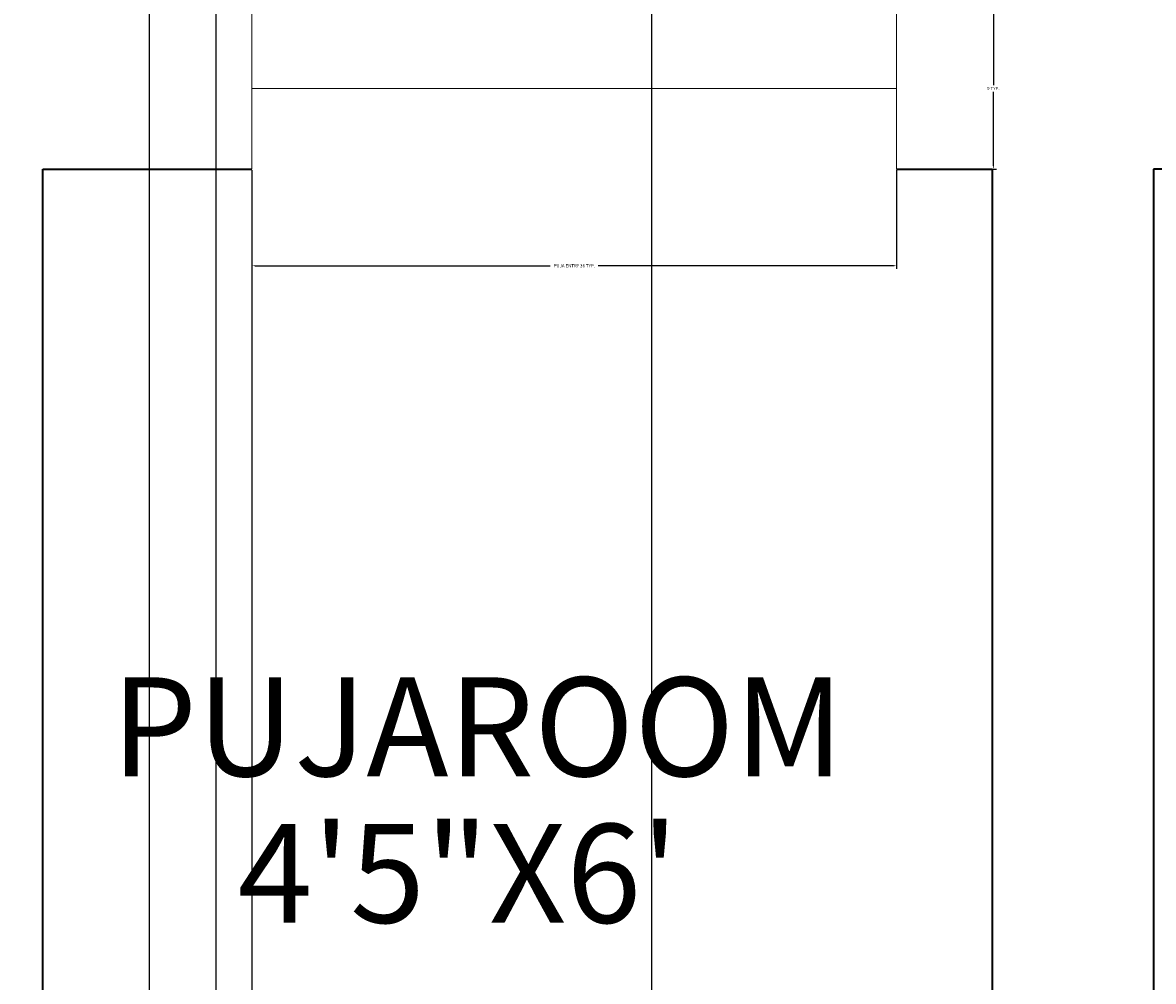
# Model space of a CAD drawing. Units: feet. Extents: x 1654 to 2985, y 1348 to 2230.
# Tile 16 of 53: x 2007 to 2070, y 1697 to 1750. Entities that reach past the tile are written whole.
import ezdxf

# ---------------------------------------------------------------- set-up
doc = ezdxf.new("R2010")
doc.units = ezdxf.units.FT
for name, color, linetype, lineweight in [('A-ANNO-DIMS', 2, 'Continuous', 18), ('A-AREA-IDEN', 7, 'Continuous', 18), ('A-WALL', 7, 'Continuous', 35), ('A-WALL-OPEN', 4, 'Continuous', 18)]:
    doc.layers.add(name, color=color, linetype=linetype, lineweight=lineweight)
doc.styles.get("Standard").update_dxf_attribs({"font": 'arial.ttf'})
doc.dimstyles.get("Standard").update_dxf_attribs({"dimtxt": 0.18, "dimasz": 0.18, "dimexe": 0.18, "dimexo": 0.0625, "dimgap": 0.09, "dimtad": 0, "dimtih": 1, "dimtoh": 1, "dimdec": 4, "dimzin": 0, "dimdsep": 46, "dimtxsty": 'Standard', "dimcen": 0.09, "dimadec": 0, "dimazin": 0, "dimtfac": 1, "dimtdec": 4, "dimtofl": 0, "dimtmove": 0, "dimatfit": 3, "dimfxl": 1, "dimtolj": 1, "dimtzin": 0, "dimarcsym": 0})

# ---------------------------------------------------------------- blocks, each defined once
blk = doc.blocks.new('OPENING-PUJA')
for p, q in [((0, 9), (0, 0)), ((36, 9), (36, 0)), ((0, 4.5), (36, 4.5))]:
    blk.add_line(p, q)
blk = doc.blocks.new('*D68')
at = {"layer": 'A-ANNO-DIMS', "color": 0, "lineweight": -2, "transparency": 16777216}
for p, q in [((2019.757, 1742.192), (2019.757, 1736.675)), ((2055.757, 1742.192), (2055.757, 1736.675)), ((2019.937, 1736.855), (2036.416, 1736.855)), ((2055.577, 1736.855), (2039.098, 1736.855))]:
    blk.add_line(p, q, dxfattribs=at)
at = {"layer": 'A-ANNO-DIMS', "color": 0, "transparency": 16777216}
for points in [[(2019.937, 1736.885), (2019.937, 1736.825), (2019.757, 1736.855)], [(2055.577, 1736.885), (2055.577, 1736.825), (2055.757, 1736.855)]]:
    blk.add_solid(points, dxfattribs=at)
at = {"layer": 'Defpoints', "color": 0, "transparency": 16777216}
for p in [(2019.757, 1742.255), (2055.757, 1742.255), (2055.757, 1736.855)]:
    blk.add_point(p, dxfattribs=at)
at = {"layer": 'A-ANNO-DIMS', "color": 0, "transparency": 16777216, "insert": (2037.757, 1736.855), "char_height": 0.18, "attachment_point": 5}
blk.add_mtext('\\A1;PUJA ENTRY 36 TYP.', dxfattribs=at)
blk = doc.blocks.new('*D69')
at = {"layer": 'A-ANNO-DIMS', "color": 0, "lineweight": -2, "transparency": 16777216}
for p, q in [((2055.819, 1751.255), (2061.337, 1751.255)), ((2061.157, 1751.075), (2061.157, 1746.937)), ((2061.157, 1742.435), (2061.157, 1746.573)), ((2055.819, 1742.255), (2061.337, 1742.255))]:
    blk.add_line(p, q, dxfattribs=at)
at = {"layer": 'A-ANNO-DIMS', "color": 0, "transparency": 16777216}
for points in [[(2061.127, 1751.075), (2061.187, 1751.075), (2061.157, 1751.255)], [(2061.127, 1742.435), (2061.187, 1742.435), (2061.157, 1742.255)]]:
    blk.add_solid(points, dxfattribs=at)
at = {"layer": 'Defpoints', "color": 0, "transparency": 16777216}
for p in [(2055.757, 1751.255), (2061.157, 1751.255), (2055.757, 1742.255)]:
    blk.add_point(p, dxfattribs=at)
at = {"layer": 'A-ANNO-DIMS', "color": 0, "transparency": 16777216, "insert": (2061.157, 1746.755), "char_height": 0.18, "attachment_point": 5}
blk.add_mtext('\\A1;9 TYP.', dxfattribs=at)
blk = doc.blocks.new('*D88')
at = {"layer": 'A-ANNO-DIMS', "color": 0, "lineweight": -2, "transparency": 16777216}
for p, q in [((2017.769, 1661.317), (2017.769, 2148.435)), ((2017.949, 2148.255), (2029.547, 2148.255)), ((2041.9, 2148.255), (2030.302, 2148.255)), ((2042.08, 1661.317), (2042.08, 2148.435))]:
    blk.add_line(p, q, dxfattribs=at)
at = {"layer": 'A-ANNO-DIMS', "color": 0, "transparency": 16777216}
for points in [[(2017.949, 2148.285), (2017.949, 2148.225), (2017.769, 2148.255)], [(2041.9, 2148.285), (2041.9, 2148.225), (2042.08, 2148.255)]]:
    blk.add_solid(points, dxfattribs=at)
at = {"layer": 'Defpoints', "color": 0, "transparency": 16777216}
for p in [(2017.769, 2148.255), (2017.769, 1661.255), (2042.08, 1661.255)]:
    blk.add_point(p, dxfattribs=at)
at = {"layer": 'A-ANNO-DIMS', "color": 0, "transparency": 16777216, "insert": (2029.925, 2148.255), "char_height": 0.18, "attachment_point": 5}
blk.add_mtext('\\A1;24.31', dxfattribs=at)
blk = doc.blocks.new('*D101')
at = {"layer": 'A-ANNO-DIMS', "color": 0, "lineweight": -2, "transparency": 16777216}
for p, q in [((1996.092, 2039.192), (1996.092, 1534.075)), ((2014.016, 2039.192), (2014.016, 1534.075)), ((1996.272, 1534.255), (2004.599, 1534.255)), ((2013.836, 1534.255), (2005.509, 1534.255))]:
    blk.add_line(p, q, dxfattribs=at)
at = {"layer": 'A-ANNO-DIMS', "color": 0, "transparency": 16777216}
for points in [[(1996.272, 1534.285), (1996.272, 1534.225), (1996.092, 1534.255)], [(2013.836, 1534.285), (2013.836, 1534.225), (2014.016, 1534.255)]]:
    blk.add_solid(points, dxfattribs=at)
at = {"layer": 'Defpoints', "color": 0, "transparency": 16777216}
for p in [(1996.092, 2039.255), (2014.016, 2039.255), (2014.016, 1534.255)]:
    blk.add_point(p, dxfattribs=at)
at = {"layer": 'A-ANNO-DIMS', "color": 0, "transparency": 16777216, "insert": (2005.054, 1534.255), "char_height": 0.18, "attachment_point": 5}
blk.add_mtext('\\A1;17.924', dxfattribs=at)
blk = doc.blocks.new('*D102')
at = {"layer": 'A-ANNO-DIMS', "color": 0, "lineweight": -2, "transparency": 16777216}
for p, q in [((2008.092, 1742.192), (2008.092, 1534.075)), ((2019.757, 1742.192), (2019.757, 1534.075)), ((2008.272, 1534.255), (2013.47, 1534.255)), ((2019.577, 1534.255), (2014.379, 1534.255))]:
    blk.add_line(p, q, dxfattribs=at)
at = {"layer": 'A-ANNO-DIMS', "color": 0, "transparency": 16777216}
for points in [[(2008.272, 1534.285), (2008.272, 1534.225), (2008.092, 1534.255)], [(2019.577, 1534.285), (2019.577, 1534.225), (2019.757, 1534.255)]]:
    blk.add_solid(points, dxfattribs=at)
at = {"layer": 'Defpoints', "color": 0, "transparency": 16777216}
for p in [(2008.092, 1742.255), (2019.757, 1742.255), (2019.757, 1534.255)]:
    blk.add_point(p, dxfattribs=at)
at = {"layer": 'A-ANNO-DIMS', "color": 0, "transparency": 16777216, "insert": (2013.925, 1534.255), "char_height": 0.18, "attachment_point": 5}
blk.add_mtext('\\A1;11.664', dxfattribs=at)

msp = doc.modelspace()

# ---------------------------------------------------------------- linework, layer by layer
at = {"layer": 'A-WALL'}
for p, q in [((2008.0924, 1670.2549), (2008.0924, 1742.2549)), ((2008.0924, 1742.2549), (2019.7567, 1742.2549)), ((2055.7567, 1742.2549), (2061.0924, 1742.2549)), ((2061.0924, 1742.2549), (2061.0924, 1670.2549)), ((2070.0924, 1742.2549), (2070.0924, 1661.2549)), ((2072.0924, 1742.2549), (2070.0924, 1742.2549))]:
    msp.add_line(p, q, dxfattribs=at)

# ---------------------------------------------------------------- block references
at = {"layer": 'A-WALL-OPEN'}
msp.add_blockref('OPENING-PUJA', (2019.757, 1742.255), dxfattribs=at)

# ---------------------------------------------------------------- texts
at = {"layer": 'A-AREA-IDEN'}
for s, p in [('PUJAROOM', (2011.9193, 1708.3501)), ('4\'5"X6\'', (2018.9644, 1700.1635))]:
    msp.add_text(s, height=5.52296, dxfattribs=at).set_placement(p)

# ---------------------------------------------------------------- dimensions: what is measured, and where the dimension line sits
at = {"layer": 'A-ANNO-DIMS'}
for base, p1, p2, override, picture, middle in [((2017.7694, 2148.2549), (2042.0798, 1661.2549), (2017.7694, 1661.2549), {"dimdec": 2, "dimlfac": 1, "dimrnd": 0, "dimzin": 0, "dimdsep": 46, "dimlunit": 2}, '*D88', (2029.9246, 2148.2549)), ((2014.016, 1534.2549), (1996.0924, 2039.2549), (2014.016, 2039.2549), {"dimdec": 3, "dimlfac": 1, "dimrnd": 0, "dimzin": 0, "dimdsep": 46, "dimlunit": 2}, '*D101', (2005.0542, 1534.2549)), ((2019.7567, 1534.2549), (2008.0924, 1742.2549), (2019.7567, 1742.2549), {"dimdec": 3, "dimlfac": 1, "dimrnd": 0, "dimzin": 0, "dimdsep": 46, "dimlunit": 2}, '*D102', (2013.9246, 1534.2549))]:
    dim = msp.add_linear_dim(base=base, p1=p1, p2=p2, dimstyle='Standard', override=override, dxfattribs=at)
    dim.commit()
    dim.dimension.update_dxf_attribs({"geometry": picture, "text_midpoint": middle})
dim = msp.add_linear_dim(base=(2061.1567, 1751.2549), p1=(2055.7567, 1742.2549), p2=(2055.7567, 1751.2549), angle=90, text='<> TYP.', dimstyle='Standard', override={"dimdec": 0, "dimlfac": 1, "dimrnd": 0, "dimzin": 0, "dimdsep": 46, "dimlunit": 2}, dxfattribs=at)
dim.commit()
dim.dimension.update_dxf_attribs({"geometry": '*D69', "text_midpoint": (2061.1567, 1746.7549)})
dim = msp.add_linear_dim(base=(2055.7567, 1736.8549), p1=(2019.7567, 1742.2549), p2=(2055.7567, 1742.2549), text='PUJA ENTRY <> TYP.', dimstyle='Standard', override={"dimdec": 0, "dimlfac": 1, "dimrnd": 0, "dimzin": 0, "dimdsep": 46, "dimlunit": 2}, dxfattribs=at)
dim.commit()
dim.dimension.update_dxf_attribs({"geometry": '*D68', "text_midpoint": (2037.7567, 1736.8549)})

doc.saveas('drawing.dxf')
